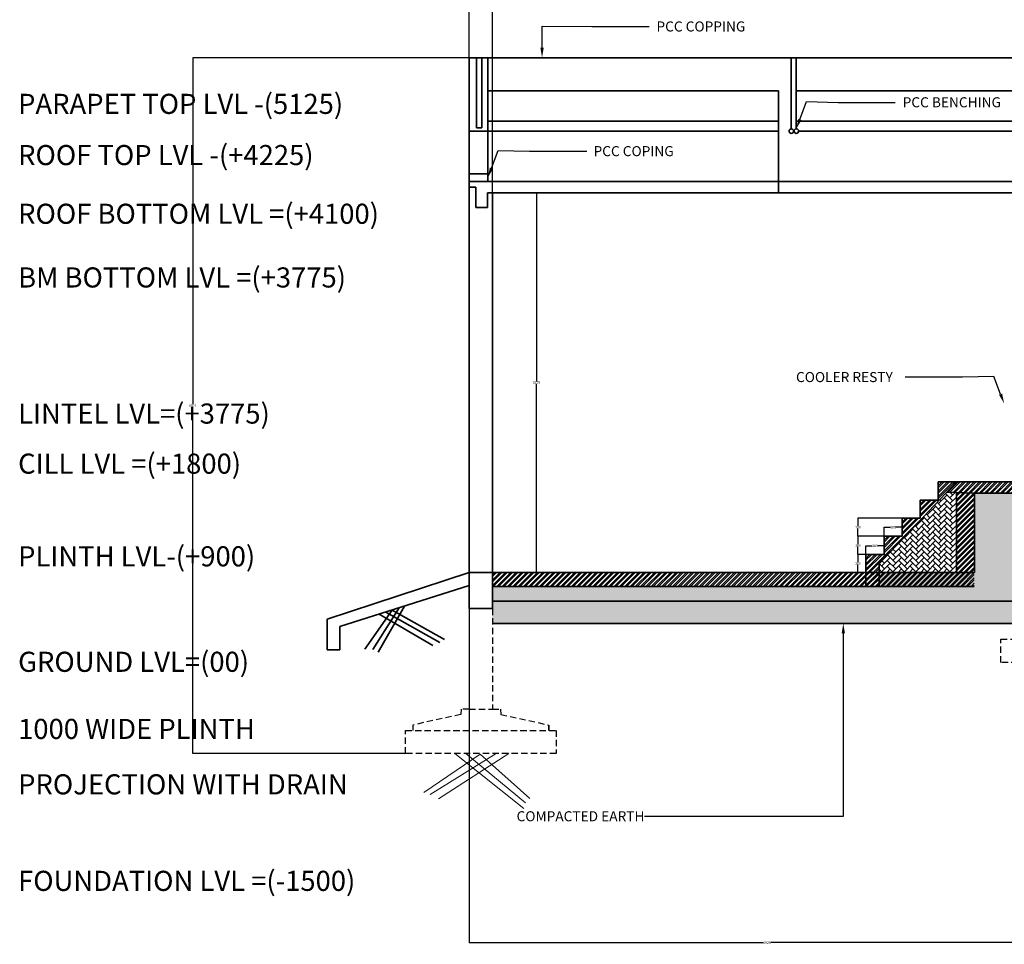
# Model space of a CAD drawing. Units: millimetres. Extents: x 1944 to 29915, y -10550 to 5909.
# Tile 1 of 24: x 1944 to 11743, y -10550 to -1353. Entities that reach past the tile are written whole.
import ezdxf
from ezdxf import colors
from ezdxf.entities.mleader import LeaderData, LeaderLine
from ezdxf.math import Vec2, Vec3

# ---------------------------------------------------------------- set-up
doc = ezdxf.new("R2010")
doc.units = ezdxf.units.MM
doc.header["$MEASUREMENT"] = 0
doc.linetypes.add('HIDDEN', pattern=[9.525, 6.35, -3.175])
for name, color, linetype, lineweight in [('A-ANNO-DIMS', 2, 'Continuous', 18), ('A-ANNO-TEXT', 7, 'Continuous', 25), ('A-FLOR-PATT', 252, 'Continuous', 13), ('A-SECT', 7, 'Continuous', 35), ('C-TOPO', 94, 'Continuous', 18), ('S-FNDN-HIDN', 1, 'HIDDEN', 25)]:
    doc.layers.add(name, color=color, linetype=linetype, lineweight=lineweight)
doc.styles.get("Standard").update_dxf_attribs({"font": 'arial.ttf'})
doc.dimstyles.get("Standard").update_dxf_attribs({"dimtxt": 25, "dimasz": 0.18, "dimexe": 0.18, "dimexo": 0.0625, "dimgap": 0.09, "dimtad": 0, "dimtih": 1, "dimtoh": 1, "dimdec": 0, "dimzin": 0, "dimdsep": 46, "dimtxsty": 'Standard', "dimcen": 0.09, "dimadec": 0, "dimazin": 0, "dimtfac": 1, "dimtdec": 0, "dimtofl": 0, "dimtmove": 0, "dimatfit": 3, "dimfxl": 1, "dimtolj": 1, "dimtzin": 0, "dimarcsym": 0})

# ---------------------------------------------------------------- blocks, each defined once
blk = doc.blocks.new('*D25')
at = {"layer": 'A-ANNO-DIMS', "color": 0, "lineweight": -2, "transparency": 16777216}
for p, q in [((6648.4, -3076), (7088, -3076)), ((7087.8, -3076.1), (7087.8, -4950.6)), ((7087.8, -6850.8), (7087.8, -4976.3)), ((6648.4, -6851), (7088, -6851))]:
    blk.add_line(p, q, dxfattribs=at)
at = {"layer": 'A-ANNO-DIMS', "color": 0, "transparency": 16777216}
for points in [[(7087.7, -3076.1), (7087.8, -3076.1), (7087.8, -3076)], [(7087.7, -6850.8), (7087.8, -6850.8), (7087.8, -6851)]]:
    blk.add_solid(points, dxfattribs=at)
at = {"layer": 'Defpoints', "color": 0, "transparency": 16777216}
for p in [(6648.3, -3076), (6648.3, -6851), (7087.8, -6851)]:
    blk.add_point(p, dxfattribs=at)
at = {"layer": 'A-ANNO-DIMS', "color": 0, "transparency": 16777216, "insert": (7087.8, -4963.5), "char_height": 25, "attachment_point": 5}
blk.add_mtext('\\A1;3775', dxfattribs=at)
blk = doc.blocks.new('*D30')
at = {"layer": 'A-ANNO-DIMS', "color": 0, "lineweight": -2, "transparency": 16777216}
for p, q in [((10365.7, -6671), (10285.4, -6671)), ((10285.6, -6671.1), (10285.6, -6748.1)), ((10365.7, -6851), (10285.4, -6851)), ((10285.6, -6850.8), (10285.6, -6773.8))]:
    blk.add_line(p, q, dxfattribs=at)
at = {"layer": 'A-ANNO-DIMS', "color": 0, "transparency": 16777216}
for points in [[(10285.6, -6671.1), (10285.6, -6671.1), (10285.6, -6671)], [(10285.6, -6850.8), (10285.6, -6850.8), (10285.6, -6851)]]:
    blk.add_solid(points, dxfattribs=at)
at = {"layer": 'Defpoints', "color": 0, "transparency": 16777216}
for p in [(10365.7, -6671), (10285.6, -6851), (10365.7, -6851)]:
    blk.add_point(p, dxfattribs=at)
at = {"layer": 'A-ANNO-DIMS', "color": 0, "transparency": 16777216, "insert": (10285.6, -6761), "char_height": 25, "attachment_point": 5}
blk.add_mtext('\\A1;180', dxfattribs=at)
blk = doc.blocks.new('*D31')
at = {"layer": 'A-ANNO-DIMS', "color": 0, "lineweight": -2, "transparency": 16777216}
for p, q in [((10365.7, -6670.9), (10365.7, -6585.2)), ((10365.9, -6585.4), (10429.3, -6585.4)), ((10545.6, -6585.4), (10482.2, -6585.4)), ((10545.7, -6670.9), (10545.7, -6585.2))]:
    blk.add_line(p, q, dxfattribs=at)
at = {"layer": 'A-ANNO-DIMS', "color": 0, "transparency": 16777216}
for points in [[(10365.9, -6585.4), (10365.9, -6585.4), (10365.7, -6585.4)], [(10545.6, -6585.4), (10545.6, -6585.4), (10545.7, -6585.4)]]:
    blk.add_solid(points, dxfattribs=at)
at = {"layer": 'Defpoints', "color": 0, "transparency": 16777216}
for p in [(10545.7, -6585.4), (10365.7, -6671), (10545.7, -6671)]:
    blk.add_point(p, dxfattribs=at)
at = {"layer": 'A-ANNO-DIMS', "color": 0, "transparency": 16777216, "insert": (10455.7, -6585.4), "char_height": 25, "attachment_point": 5}
blk.add_mtext('\\A1;180', dxfattribs=at)
blk = doc.blocks.new('*D32')
at = {"layer": 'A-ANNO-DIMS', "color": 0, "lineweight": -2, "transparency": 16777216}
for p, q in [((10545.7, -6491), (10285.4, -6491)), ((10285.6, -6491.1), (10285.6, -6568.1)), ((10285.6, -6670.8), (10285.6, -6593.8)), ((10545.7, -6671), (10285.4, -6671))]:
    blk.add_line(p, q, dxfattribs=at)
at = {"layer": 'A-ANNO-DIMS', "color": 0, "transparency": 16777216}
for points in [[(10285.6, -6491.1), (10285.6, -6491.1), (10285.6, -6491)], [(10285.6, -6670.8), (10285.6, -6670.8), (10285.6, -6671)]]:
    blk.add_solid(points, dxfattribs=at)
at = {"layer": 'Defpoints', "color": 0, "transparency": 16777216}
for p in [(10545.7, -6491), (10285.6, -6671), (10545.7, -6671)]:
    blk.add_point(p, dxfattribs=at)
at = {"layer": 'A-ANNO-DIMS', "color": 0, "transparency": 16777216, "insert": (10285.6, -6581), "char_height": 25, "attachment_point": 5}
blk.add_mtext('\\A1;180', dxfattribs=at)
blk = doc.blocks.new('*D33')
at = {"layer": 'A-ANNO-DIMS', "color": 0, "lineweight": -2, "transparency": 16777216}
for p, q in [((10545.7, -6490.9), (10545.7, -6400.4)), ((10545.9, -6400.6), (10609.3, -6400.6)), ((10725.6, -6400.6), (10662.2, -6400.6)), ((10725.7, -6490.9), (10725.7, -6400.4))]:
    blk.add_line(p, q, dxfattribs=at)
at = {"layer": 'A-ANNO-DIMS', "color": 0, "transparency": 16777216}
for points in [[(10545.9, -6400.6), (10545.9, -6400.6), (10545.7, -6400.6)], [(10725.6, -6400.6), (10725.6, -6400.6), (10725.7, -6400.6)]]:
    blk.add_solid(points, dxfattribs=at)
at = {"layer": 'Defpoints', "color": 0, "transparency": 16777216}
for p in [(10725.7, -6400.6), (10545.7, -6491), (10725.7, -6491)]:
    blk.add_point(p, dxfattribs=at)
at = {"layer": 'A-ANNO-DIMS', "color": 0, "transparency": 16777216, "insert": (10635.7, -6400.6), "char_height": 25, "attachment_point": 5}
blk.add_mtext('\\A1;180', dxfattribs=at)
blk = doc.blocks.new('*D34')
at = {"layer": 'A-ANNO-DIMS', "color": 0, "lineweight": -2, "transparency": 16777216}
for p, q in [((10725.7, -6311), (10285.4, -6311)), ((10285.6, -6311.1), (10285.6, -6388.1)), ((10285.6, -6490.8), (10285.6, -6413.8)), ((10725.7, -6491), (10285.4, -6491))]:
    blk.add_line(p, q, dxfattribs=at)
at = {"layer": 'A-ANNO-DIMS', "color": 0, "transparency": 16777216}
for points in [[(10285.6, -6311.1), (10285.6, -6311.1), (10285.6, -6311)], [(10285.6, -6490.8), (10285.6, -6490.8), (10285.6, -6491)]]:
    blk.add_solid(points, dxfattribs=at)
at = {"layer": 'Defpoints', "color": 0, "transparency": 16777216}
for p in [(10725.7, -6311), (10285.6, -6491), (10725.7, -6491)]:
    blk.add_point(p, dxfattribs=at)
at = {"layer": 'A-ANNO-DIMS', "color": 0, "transparency": 16777216, "insert": (10285.6, -6401), "char_height": 25, "attachment_point": 5}
blk.add_mtext('\\A1;180', dxfattribs=at)
blk = doc.blocks.new('EARTH-COMPACT-SYMB')
for q in [(0, 60.9), (1053, 0)]:
    blk.add_line((559.8, 441.1), q)
blk = doc.blocks.new('*D85')
at = {"layer": 'A-ANNO-DIMS', "color": 0, "lineweight": -2, "transparency": 16777216}
for p, q in [((6418.3, -1730.7), (6418.3, -395.6)), ((6418.5, -395.8), (15860.3, -395.8)), ((25389.1, -395.8), (15947.3, -395.8)), ((25389.3, -1846.5), (25389.3, -395.6))]:
    blk.add_line(p, q, dxfattribs=at)
at = {"layer": 'A-ANNO-DIMS', "color": 0, "transparency": 16777216}
for points in [[(6418.5, -395.7), (6418.5, -395.8), (6418.3, -395.8)], [(25389.1, -395.7), (25389.1, -395.8), (25389.3, -395.8)]]:
    blk.add_solid(points, dxfattribs=at)
at = {"layer": 'Defpoints', "color": 0, "transparency": 16777216}
for p in [(25389.3, -395.8), (6418.3, -1730.8), (25389.3, -1846.5)]:
    blk.add_point(p, dxfattribs=at)
at = {"layer": 'A-ANNO-DIMS', "color": 0, "transparency": 16777216, "insert": (15903.8, -395.8), "char_height": 25, "attachment_point": 5}
blk.add_mtext('\\A1;18971', dxfattribs=at)
blk = doc.blocks.new('*D86')
at = {"layer": 'A-ANNO-DIMS', "color": 0, "lineweight": -2, "transparency": 16777216}
for p, q in [((12344, -6305.8), (12344, -10533.3)), ((6418.3, -6851), (6418.3, -10533.3)), ((6418.5, -10533.1), (9343.7, -10533.1)), ((12343.8, -10533.1), (9418.6, -10533.1))]:
    blk.add_line(p, q, dxfattribs=at)
at = {"layer": 'A-ANNO-DIMS', "color": 0, "transparency": 16777216}
for points in [[(6418.5, -10533.1), (6418.5, -10533.1), (6418.3, -10533.1)], [(12343.8, -10533.1), (12343.8, -10533.1), (12344, -10533.1)]]:
    blk.add_solid(points, dxfattribs=at)
at = {"layer": 'Defpoints', "color": 0, "transparency": 16777216}
for p in [(12344, -6305.8), (6418.3, -6851), (12344, -10533.1)]:
    blk.add_point(p, dxfattribs=at)
at = {"layer": 'A-ANNO-DIMS', "color": 0, "transparency": 16777216, "insert": (9381.1, -10533.1), "char_height": 25, "attachment_point": 5}
blk.add_mtext('\\A1;5926', dxfattribs=at)
blk = doc.blocks.new('*D90')
at = {"layer": 'A-ANNO-DIMS', "color": 0, "lineweight": -2, "transparency": 16777216}
for p, q in [((6418.3, -3019.9), (6418.3, -395.6)), ((6418.5, -395.8), (6505.4, -395.8)), ((6648.1, -395.8), (6561.2, -395.8)), ((6648.3, -3075.9), (6648.3, -395.6))]:
    blk.add_line(p, q, dxfattribs=at)
at = {"layer": 'A-ANNO-DIMS', "color": 0, "transparency": 16777216}
for points in [[(6418.5, -395.7), (6418.5, -395.8), (6418.3, -395.8)], [(6648.1, -395.7), (6648.1, -395.8), (6648.3, -395.8)]]:
    blk.add_solid(points, dxfattribs=at)
at = {"layer": 'Defpoints', "color": 0, "transparency": 16777216}
for p in [(6648.3, -395.8), (6418.3, -3020), (6648.3, -3076)]:
    blk.add_point(p, dxfattribs=at)
at = {"layer": 'A-ANNO-DIMS', "color": 0, "transparency": 16777216, "insert": (6533.3, -395.8), "char_height": 25, "attachment_point": 5}
blk.add_mtext('\\A1;230', dxfattribs=at)
blk = doc.blocks.new('*D99')
at = {"layer": 'A-ANNO-DIMS', "color": 0, "lineweight": -2, "transparency": 16777216}
for p, q in [((6418.3, -1730.8), (3668.1, -1730.8)), ((3668.3, -1730.9), (3668.3, -5178.2)), ((3668.3, -8651.3), (3668.3, -5203.9)), ((5783.3, -8651.4), (3668.1, -8651.4))]:
    blk.add_line(p, q, dxfattribs=at)
at = {"layer": 'A-ANNO-DIMS', "color": 0, "transparency": 16777216}
for points in [[(3668.3, -1730.9), (3668.4, -1730.9), (3668.3, -1730.8)], [(3668.3, -8651.3), (3668.4, -8651.3), (3668.3, -8651.4)]]:
    blk.add_solid(points, dxfattribs=at)
at = {"layer": 'Defpoints', "color": 0, "transparency": 16777216}
for p in [(3668.3, -1730.8), (6418.3, -1730.8), (5783.3, -8651.4)]:
    blk.add_point(p, dxfattribs=at)
at = {"layer": 'A-ANNO-DIMS', "color": 0, "transparency": 16777216, "insert": (3668.3, -5191.1), "char_height": 25, "attachment_point": 5}
blk.add_mtext('\\A1;6921', dxfattribs=at)

msp = doc.modelspace()

# ---------------------------------------------------------------- hatches: boundary and pattern name
at = {"layer": 'A-FLOR-PATT'}
h = msp.add_hatch(dxfattribs=at)
h.set_pattern_fill('ANSI32', color=256, scale=100)
h.paths.add_polyline_path([(11265.739, -5950.967), (11085.739, -5950.967), (11085.739, -6130.967), (10905.739, -6130.967), (10905.739, -6310.967), (10725.739, -6310.967), (10725.739, -6490.967), (10545.739, -6490.967), (10545.739, -6670.967), (10365.739, -6670.967), (10365.739, -6850.967), (10365.739, -6990.545), (10496.11, -6990.545), (10496.11, -6763.893)], flags=17)
h = msp.add_hatch(dxfattribs=at)
h.set_pattern_fill('ANSI32', color=256, scale=100)
h.paths.add_polyline_path([(12343.981, -5950.967), (11265.739, -5950.967), (11169.087, -6053.056), (11445.739, -6061.05), (12343.981, -6061.05)])
h = msp.add_hatch(dxfattribs=at)
h.set_pattern_fill('AR-HBONE', color=256, scale=10)
h.paths.add_polyline_path([(12343.981, -6305.752), (12343.981, -6061.05), (11445.739, -6061.05), (11445.739, -6850.967), (11265.739, -6850.967), (10496.11, -6850.967), (10496.11, -6990.545), (6648.315, -6990.545), (6648.315, -7135.877), (12343.981, -7135.877)])
h = msp.add_hatch(dxfattribs=at)
h.set_pattern_fill('AR-HBONE', color=256, scale=10)
h.paths.add_polyline_path([(11265.739, -6055.849), (11169.087, -6053.056), (10496.11, -6763.893), (10496.11, -6850.967), (11265.739, -6850.967)])
h = msp.add_hatch(dxfattribs=at)
h.set_pattern_fill('ANSI32', color=256, scale=100)
h.paths.add_polyline_path([(11445.739, -6061.05), (11265.739, -6055.849), (11265.739, -6850.967), (11445.739, -6850.967)])
h = msp.add_hatch(dxfattribs=at)
h.set_pattern_fill('ANSI32', color=256, scale=100)
h.paths.add_polyline_path([(11443.981, -6850.967), (6648.315, -6850.967), (6648.315, -6990.545), (11443.981, -6990.545)])
h = msp.add_hatch(dxfattribs=at)
h.set_pattern_fill('AR-HBONE', color=256, scale=10)
h.paths.add_polyline_path([(12343.981, -7135.877), (6648.315, -7135.877), (6648.315, -7210.967), (6648.315, -7357.264), (12261.31, -7357.264), (12261.952, -7304.748), (12343.981, -7305.752)])

# ---------------------------------------------------------------- linework, layer by layer
at = {"layer": 'A-SECT'}
for p, q in [((6418.315, -1730.752), (16516.552, -1730.752)), ((6418.315, -2060.967), (6418.315, -1730.752)), ((6490.876, -1730.752), (6490.876, -2427.886)), ((6542.801, -2427.886), (6542.801, -1730.752)), ((6602.753, -2887.759), (6602.753, -1730.752)), ((9622.957, -2439.295), (9622.957, -1730.752)), ((9672.957, -2438.351), (9672.957, -1730.752)), ((6418.315, -2060.967), (6418.315, -2960.967)), ((6602.753, -2060.967), (9496.148, -2060.967)), ((9496.148, -3075.967), (9496.148, -2060.967)), ((9672.957, -2060.967), (16516.552, -2060.967)), ((6490.876, -2427.886), (6542.801, -2427.886)), ((6602.753, -2360.967), (9496.148, -2360.967)), ((9672.957, -2360.967), (16516.552, -2360.967)), ((6418.315, -2460.967), (9496.148, -2460.967)), ((9695.572, -2460.967), (16516.552, -2460.967)), ((6418.315, -2960.967), (6418.315, -2887.759)), ((6418.315, -2887.759), (6602.753, -2887.759)), ((6602.753, -2887.759), (6602.753, -2960.967)), ((6418.315, -2960.967), (6418.315, -6850.967)), ((6418.315, -2960.967), (12343.981, -2960.967)), ((6418.315, -3019.985), (6482.851, -3019.985)), ((6482.851, -3019.985), (6482.851, -3219.543)), ((6599.177, -3219.543), (6599.177, -3075.967)), ((6599.177, -3075.967), (6648.315, -3075.967)), ((6648.315, -3075.967), (6648.315, -6850.967)), ((6648.315, -3075.967), (12343.981, -3075.967)), ((6482.851, -3219.543), (6599.177, -3219.543)), ((10496.11, -6763.893), (11265.739, -5950.967)), ((11085.739, -6130.967), (11085.739, -5950.967)), ((11085.739, -5950.967), (11265.739, -5950.967)), ((12343.981, -5950.967), (11265.739, -5950.967)), ((11445.739, -6061.05), (11169.087, -6053.056)), ((11265.739, -6055.849), (11265.739, -6850.967)), ((11445.739, -6850.967), (11445.739, -6061.05)), ((11445.739, -6061.05), (12343.981, -6061.05)), ((10905.739, -6310.967), (10905.739, -6130.967)), ((10905.739, -6130.967), (11085.739, -6130.967)), ((10725.739, -6490.967), (10725.739, -6310.967)), ((10725.739, -6310.967), (10905.739, -6310.967)), ((10545.739, -6670.967), (10545.739, -6490.967)), ((10545.739, -6490.967), (10725.739, -6490.967)), ((10365.739, -6850.967), (10365.739, -6670.967)), ((10365.739, -6670.967), (10545.739, -6670.967)), ((6418.315, -6850.967), (5003.329, -7316.598)), ((6648.315, -6850.967), (11443.981, -6850.967)), ((10365.739, -6850.967), (10365.739, -6990.545)), ((10496.11, -6990.545), (10496.11, -6763.893)), ((11265.739, -6850.967), (11445.739, -6850.967)), ((5130.252, -7389.626), (6418.315, -6982.208)), ((11443.981, -6990.545), (6648.315, -6990.545)), ((10365.739, -6990.545), (10496.11, -6990.545)), ((6648.315, -7135.877), (12343.981, -7135.877)), ((5649.78, -7225.298), (5380.251, -7612.552)), ((5380.251, -7612.552), (5649.78, -7225.298)), ((5721.918, -7202.48), (5457.174, -7616.396)), ((5774.283, -7185.917), (5512.532, -7644.029)), ((5588.544, -7244.667), (6125.596, -7547.471)), ((5649.78, -7225.298), (6172.558, -7516.463)), ((5003.329, -7316.598), (5003.329, -7620.239)), ((5521.133, -7265.989), (6054.254, -7579.006)), ((5130.252, -7620.239), (5130.252, -7389.626)), ((12261.31, -7357.264), (6648.315, -7357.264)), ((5003.329, -7620.239), (5130.252, -7620.239)), ((7210.939, -8368.553), (7210.939, -8421.433))]:
    msp.add_line(p, q, dxfattribs=at)
msp.add_lwpolyline([(6418.315, -6850.967), (6648.315, -6850.967), (6648.315, -7210.967), (6418.315, -7210.967)], close=True, dxfattribs=at)
for centre in [(9622.957, -2461.91), (9672.957, -2460.967)]:
    msp.add_circle(centre, 22.615, dxfattribs=at)
at = {"layer": 'C-TOPO'}
for p, q in [((6686.219, -8651.433), (6027.921, -9061.062)), ((6811.174, -8651.433), (6111.733, -9102.178)), ((6273.259, -8651.433), (6962.034, -9198.115)), ((6384.5, -8651.433), (6977.273, -9143.294))]:
    msp.add_line(p, q, dxfattribs=at)
at = {"layer": 'S-FNDN-HIDN', "ltscale": 10}
for p, q in [((6418.315, -7210.967), (6418.315, -8210.967)), ((6648.315, -7210.967), (6648.315, -8210.967)), ((6336.286, -8209.963), (6335.644, -8262.478)), ((6418.315, -8210.967), (6336.286, -8209.963)), ((6418.315, -8210.967), (6648.315, -8210.967)), ((6648.315, -8210.967), (6730.344, -8209.963)), ((6730.344, -8209.963), (6730.986, -8262.478)), ((6335.644, -8262.478), (5855.691, -8368.553)), ((6730.986, -8262.478), (7210.939, -8368.553)), ((5855.691, -8368.553), (5855.691, -8421.433))]:
    msp.add_line(p, q, dxfattribs=at)
for points in [[(11708.981, -7516.218), (13208.981, -7516.218), (13208.981, -7746.218), (11708.981, -7746.218)], [(5783.315, -8421.433), (7283.315, -8421.433), (7283.315, -8651.433), (5783.315, -8651.433)]]:
    msp.add_lwpolyline(points, close=True, dxfattribs=at)

# ---------------------------------------------------------------- block references
at = {"layer": 'C-TOPO'}
msp.add_blockref('EARTH-COMPACT-SYMB', (5966.968, -9099.132), dxfattribs=at)

# ---------------------------------------------------------------- texts
at = {"layer": 'A-ANNO-TEXT'}
for s, p in [('PARAPET TOP LVL -(5125)', (1928.442, -2290.286)), ('ROOF TOP LVL -(+4225)', (1928.442, -2799.551)), ('ROOF BOTTOM LVL =(+4100)', (1928.442, -3383.343)), ('BM BOTTOM LVL =(+3775)', (1928.442, -4016.82)), ('LINTEL LVL=(+3775)', (1928.442, -5370.721)), ('CILL LVL =(+1800)', (1928.442, -5868.7)), ('PLINTH LVL-(+900)', (1928.442, -6790.568)), ('GROUND LVL=(00)', (1928.442, -7839.589)), ('1000 WIDE PLINTH ', (1928.442, -8507.149)), ('PROJECTION WITH DRAIN', (1928.442, -9058.579)), ('FOUNDATION LVL =(-1500)', (1928.442, -10018.477))]:
    msp.add_text(s, height=200, dxfattribs=at).set_placement(p)

# ---------------------------------------------------------------- dimensions: what is measured, and where the dimension line sits
at = {"layer": 'A-ANNO-DIMS'}
for base, p1, p2, override, picture, middle in [((25389.297, -395.752), (6418.315, -1730.752), (25389.297, -1846.542), {"dimdec": 0, "dimlfac": 1, "dimrnd": 0, "dimzin": 0, "dimdsep": 46, "dimlunit": 2}, '*D85', (15903.806, -395.752)), ((6648.315, -395.752), (6418.315, -3019.985), (6648.315, -3075.967), {"dimdec": 0, "dimlfac": 1, "dimrnd": 0, "dimzin": 0, "dimdsep": 46, "dimlunit": 2}, '*D90', (6533.315, -395.752)), ((12343.981, -10533.115), (6418.315, -6850.967), (12343.981, -6305.752), {"dimdec": 0, "dimlfac": 1, "dimrnd": 0, "dimzin": 0, "dimdsep": 46, "dimlunit": 2}, '*D86', (9381.148, -10533.115)), ((10725.739, -6400.584), (10545.739, -6490.967), (10725.739, -6490.967), {"dimclrd": 0, "dimclre": 0, "dimclrt": 0}, '*D33', (10635.739, -6400.584)), ((10545.739, -6585.409), (10365.739, -6670.967), (10545.739, -6670.967), {"dimclrd": 0, "dimclre": 0, "dimclrt": 0}, '*D31', (10455.739, -6585.409))]:
    dim = msp.add_linear_dim(base=base, p1=p1, p2=p2, dimstyle='Standard', override=override, dxfattribs=at)
    dim.commit()
    dim.dimension.update_dxf_attribs({"geometry": picture, "text_midpoint": middle})
for base, p1, p2, override, picture, middle in [((3668.329, -1730.752), (5783.315, -8651.433), (6418.315, -1730.752), {"dimdec": 0, "dimlfac": 1, "dimrnd": 0, "dimzin": 0, "dimdsep": 46, "dimlunit": 2}, '*D99', (3668.329, -5191.092)), ((7087.775, -6850.967), (6648.315, -3075.967), (6648.315, -6850.967), {"dimclrd": 0, "dimclre": 0, "dimclrt": 0}, '*D25', (7087.775, -4963.467)), ((10285.608, -6490.967), (10725.739, -6310.967), (10725.739, -6490.967), {"dimclrd": 0, "dimclre": 0, "dimclrt": 0}, '*D34', (10285.608, -6400.967)), ((10285.608, -6670.967), (10545.739, -6490.967), (10545.739, -6670.967), {"dimclrd": 0, "dimclre": 0, "dimclrt": 0}, '*D32', (10285.608, -6580.967)), ((10285.608, -6850.967), (10365.739, -6670.967), (10365.739, -6850.967), {"dimclrd": 0, "dimclre": 0, "dimclrt": 0}, '*D30', (10285.608, -6760.967))]:
    dim = msp.add_linear_dim(base=base, p1=p1, p2=p2, angle=90, dimstyle='Standard', override=override, dxfattribs=at)
    dim.commit()
    dim.dimension.update_dxf_attribs({"geometry": picture, "text_midpoint": middle})

# ---------------------------------------------------------------- leaders
at = {"layer": 'A-ANNO-TEXT'}
ml = msp.add_multileader_mtext('Standard', dxfattribs=at)
ml.set_content('PCC COPPING', color=256)
ml.set_leader_properties()
ml.build(insert=Vec2(0, 0))
ml.multileader.update_dxf_attribs({"dogleg_length": 568.936, "arrow_head_size": 100})
ctx = ml.context
ctx.base_point, ctx.char_height, ctx.arrow_head_size, ctx.landing_gap_size, ctx.plane_origin = Vec3(8206.955, -1421.356), 100, 100, 0.09, Vec3(7638.019, -1421.356)
ctx.text_align_type = 2
notes = []
notes.append((ctx, [(0, (1, 1, 0), (7638.019, -1421.356), (1, 0), 568.936, [(0, [(7142.635, -1730.752), (7142.635, -1416.503)], 0, [])])]))
ctx.mtext.insert, ctx.mtext.alignment, ctx.mtext.flow_direction = Vec3(9165.572, -1370.503), 3, 5
ml = msp.add_multileader_mtext('Standard', dxfattribs=at)
ml.set_content('PCC BENCHING', color=256)
ml.set_leader_properties()
ml.build(insert=Vec2(0, 0))
ml.multileader.update_dxf_attribs({"dogleg_length": 568.936, "arrow_head_size": 100})
ctx = ml.context
ctx.base_point, ctx.char_height, ctx.arrow_head_size, ctx.landing_gap_size, ctx.plane_origin = Vec3(10657.907, -2175.407), 100, 100, 0.09, Vec3(10088.971, -2175.407)
ctx.text_align_type = 2
notes.append((ctx, [(0, (1, 1, 0), (10088.971, -2175.407), (1, 0), 568.936, [(0, [(9672.957, -2438.351), (9775.735, -2168.12)], 0, [])])]))
ctx.mtext.insert, ctx.mtext.alignment, ctx.mtext.flow_direction = Vec3(11709.634, -2124.554), 3, 5
ml = msp.add_multileader_mtext('Standard', dxfattribs=at)
ml.set_content('PCC COPING', color=256)
ml.set_leader_properties()
ml.build(insert=Vec2(0, 0))
ml.multileader.update_dxf_attribs({"dogleg_length": 568.936, "arrow_head_size": 100})
ctx = ml.context
ctx.base_point, ctx.char_height, ctx.arrow_head_size, ctx.landing_gap_size, ctx.plane_origin = Vec3(7587.702, -2661.418), 100, 100, 0.09, Vec3(7018.767, -2661.418)
ctx.text_align_type = 2
notes.append((ctx, [(0, (1, 1, 0), (7018.767, -2661.418), (1, 0), 568.936, [(0, [(6602.753, -2924.363), (6705.531, -2654.131)], 0, [])])]))
ctx.mtext.insert, ctx.mtext.alignment, ctx.mtext.flow_direction = Vec3(8453.14, -2610.566), 3, 5
ml = msp.add_multileader_mtext('Standard', dxfattribs=at)
ml.set_content('COOLER RESTY', color=256)
ml.set_leader_properties()
ml.build(insert=Vec2(0, 0))
ml.multileader.update_dxf_attribs({"dogleg_length": 568.936, "arrow_head_size": 100})
ctx = ml.context
ctx.base_point, ctx.char_height, ctx.arrow_head_size, ctx.landing_gap_size, ctx.plane_origin = Vec3(9669.818, -4908.567), 100, 100, 0.09, Vec3(11325.428, -4908.567)
notes.append((ctx, [(0, (1, 1, 0), (11325.428, -4908.567), (-1, 0), 568.936, [(0, [(11741.442, -5171.512), (11638.664, -4901.28)], 0, [])])]))
ctx.mtext.insert, ctx.mtext.flow_direction = Vec3(9669.908, -4857.715), 5
ml = msp.add_multileader_mtext('Standard', dxfattribs=at)
ml.set_content('COMPACTED EARTH ', color=256)
ml.set_leader_properties()
ml.build(insert=Vec2(0, 0))
ml.multileader.update_dxf_attribs({"dogleg_length": 568.936, "arrow_head_size": 100})
ctx = ml.context
ctx.base_point, ctx.char_height, ctx.arrow_head_size, ctx.landing_gap_size, ctx.plane_origin = Vec3(6775.18, -9276.85), 100, 100, 0.09, Vec3(8730.926, -9276.85)
ctx.text_align_type = 2
notes.append((ctx, [(0, (1, 1, 0), (8730.926, -9276.85), (-1, 0), 568.936, [(0, [(10140.433, -7357.264), (10140.433, -9276.85)], 0, [])])]))
ctx.mtext.insert, ctx.mtext.alignment, ctx.mtext.flow_direction = Vec3(8161.901, -9225.997), 3, 5
for ctx, leaders in notes:
    for number, flags, end, landing, length, lines in leaders:
        leader = LeaderData()
        leader.index, (leader.has_last_leader_line, leader.has_dogleg_vector, leader.attachment_direction) = number, flags
        leader.last_leader_point, leader.dogleg_vector, leader.dogleg_length = Vec3(end), Vec3(landing), length
        for number, points, colour, breaks in lines:
            line = LeaderLine()
            line.index, line.vertices, line.color, line.breaks = number, Vec3.list(points), colors.encode_raw_color(colour), breaks
            leader.lines.append(line)
        ctx.leaders.append(leader)

doc.saveas('drawing.dxf')
